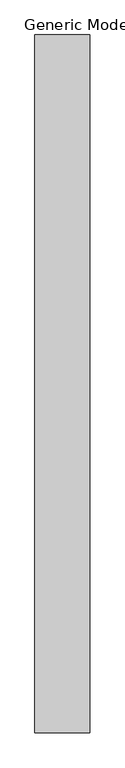
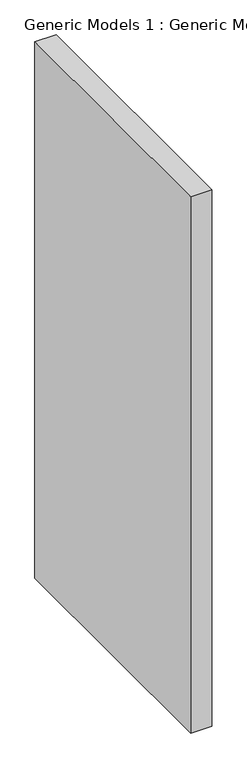
"""IFC4 building model written with IfcOpenShell, lengths in millimetres: proxy geometry, Generic Models 1 : Generic Models 1."""

from ifc_helpers import new_model, si_unit, frame, origin, place, context, project, spatial, polyline, outline, extrude, source, transform, mapped, element, save


def generic_models_1_generic_models_1_1482fe98(model_context):
    return source(origin(), model_context, "Body", "SweptSolid", [
        extrude(outline(polyline([(1894.6218735, -7288.8014349), (1666.0218735, -7288.8014349), (1666.0218735, -4389.2142532), (1894.6218735, -4389.2142532), (1894.6218735, -7288.8014349)])), frame((0.0, 0.0, 3345.9887369), z_axis=(0.0, 0.0, 1.0), x_axis=(1.0, 0.0, 0.0)), (0.0, 0.0, 1.0), 6101.2240725),
    ])


if __name__ == "__main__":
    model = new_model("IFC4")
    model_context = context("Model", 3, world=origin())
    ifc_project = project(units=[si_unit("LENGTHUNIT", "METRE", prefix="MILLI")], contexts=[model_context])
    site = spatial("IfcSite", under=ifc_project)
    building = spatial("IfcBuilding", under=site)
    placement = place(None, origin())
    generic_models_1_generic_models_1_shape = generic_models_1_generic_models_1_1482fe98(model_context)
    element("IfcBuildingElementProxy", 1, Name="Generic Models 1 : Generic Models 1", ObjectType="Generic Models 1 : Generic Models 1", at=placement, inside=building, context=model_context, shape_type="MappedRepresentation", body=[
        mapped(generic_models_1_generic_models_1_shape, transform((0.0, 0.0, 0.0), x_axis=(1.0, 0.0, 0.0), y_axis=(0.0, 1.0, 0.0), z_axis=(0.0, 0.0, 1.0))),
    ])
    save(model, "model.ifc")

# Revit data of these elements
# Element 1 (IfcBuildingElementProxy, "Generic Models 1 : Generic Models 1")
#   Materials on its faces: "WALL PAINT"
# Materials
#   "WALL PAINT": class "Generic", colour RGB 120 120 120, transparency 0, Cost = 0
